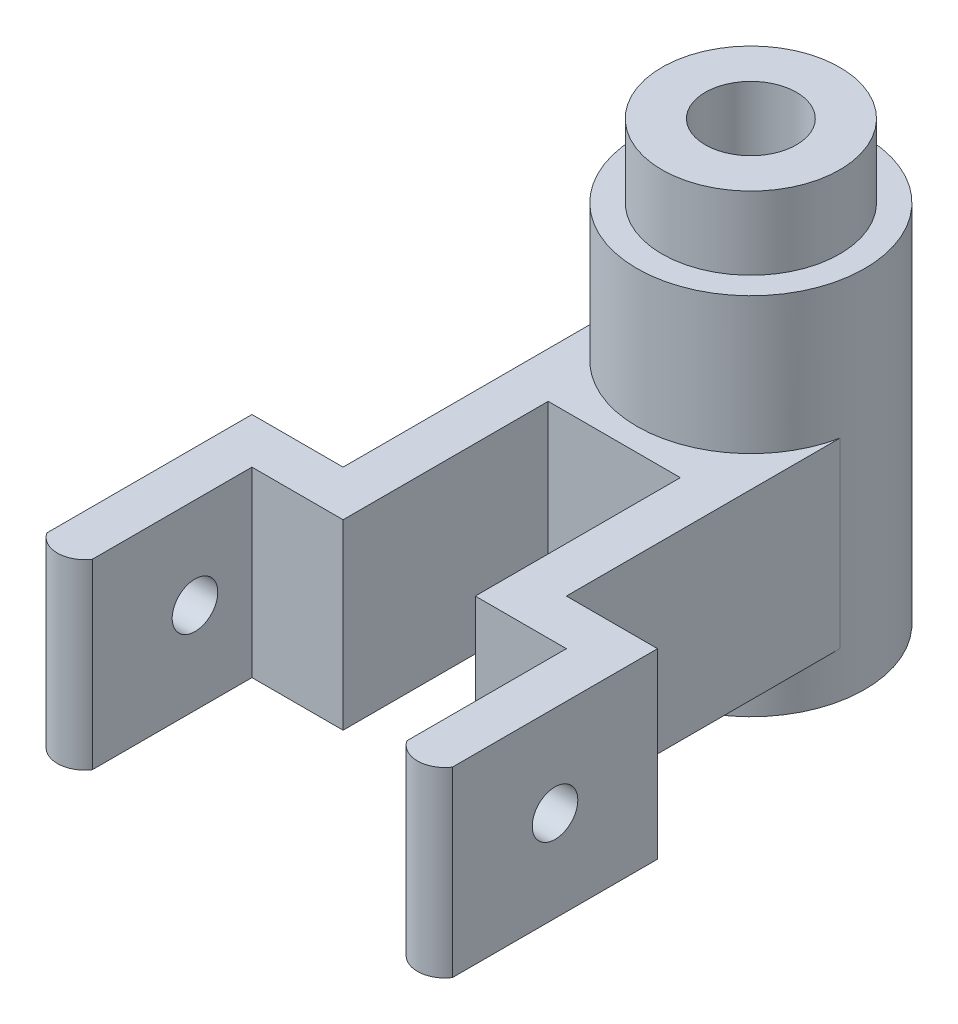
ISO-10303-21;
HEADER;
FILE_DESCRIPTION(('STEP AP214'),'2;1');
FILE_NAME('part.step','',(''),(''),'','','');
FILE_SCHEMA(('AUTOMOTIVE_DESIGN { 1 0 10303 214 1 1 1 1 }'));
ENDSEC;
DATA;
#1=APPLICATION_CONTEXT('core data for automotive mechanical design processes');
#2=APPLICATION_PROTOCOL_DEFINITION('international standard','automotive_design',2000,#1);
#3=PRODUCT_CONTEXT('',#1,'mechanical');
#4=PRODUCT('Part','Part','',(#3));
#5=PRODUCT_RELATED_PRODUCT_CATEGORY('part','',(#4));
#6=PRODUCT_DEFINITION_FORMATION('','',#4);
#7=PRODUCT_DEFINITION_CONTEXT('part definition',#1,'design');
#8=PRODUCT_DEFINITION('design','',#6,#7);
#9=PRODUCT_DEFINITION_SHAPE('','',#8);
#10=(LENGTH_UNIT() NAMED_UNIT(*) SI_UNIT(.MILLI.,.METRE.));
#11=(NAMED_UNIT(*) PLANE_ANGLE_UNIT() SI_UNIT($,.RADIAN.));
#12=(NAMED_UNIT(*) SI_UNIT($,.STERADIAN.) SOLID_ANGLE_UNIT());
#13=UNCERTAINTY_MEASURE_WITH_UNIT(LENGTH_MEASURE(1.E-05),#10,'distance_accuracy_value','');
#14=(GEOMETRIC_REPRESENTATION_CONTEXT(3) GLOBAL_UNCERTAINTY_ASSIGNED_CONTEXT((#13)) GLOBAL_UNIT_ASSIGNED_CONTEXT((#10,
#11,#12)) REPRESENTATION_CONTEXT('',''));
#15=CARTESIAN_POINT('',(0.,0.,0.));
#16=DIRECTION('',(0.,0.,1.));
#17=DIRECTION('',(1.,0.,0.));
#18=AXIS2_PLACEMENT_3D('',#15,#16,#17);
#19=CARTESIAN_POINT('',(0.,80.,0.));
#20=DIRECTION('',(0.,-1.,0.));
#21=DIRECTION('',(0.,0.,-1.));
#22=AXIS2_PLACEMENT_3D('',#19,#20,#21);
#23=CYLINDRICAL_SURFACE('',#22,25.);
#24=DIRECTION('',(0.,-1.,0.));
#25=VECTOR('',#24,1.);
#26=CARTESIAN_POINT('',(-24.5,50.,4.97493718553311));
#27=LINE('',#26,#25);
#28=CARTESIAN_POINT('',(-24.5,50.,4.97493718553311));
#29=VERTEX_POINT('',#28);
#30=CARTESIAN_POINT('',(-24.5,9.99999999999999,4.97493718553311));
#31=VERTEX_POINT('',#30);
#32=EDGE_CURVE('E60',#29,#31,#27,.T.);
#33=ORIENTED_EDGE('',*,*,#32,.F.);
#34=CARTESIAN_POINT('',(0.,50.,0.));
#35=DIRECTION('',(0.,1.,0.));
#36=DIRECTION('',(0.,0.,1.));
#37=AXIS2_PLACEMENT_3D('',#34,#35,#36);
#38=CIRCLE('',#37,25.);
#39=CARTESIAN_POINT('',(24.5,50.,4.97493718553311));
#40=VERTEX_POINT('',#39);
#41=EDGE_CURVE('E63',#29,#40,#38,.T.);
#42=ORIENTED_EDGE('',*,*,#41,.T.);
#43=DIRECTION('',(0.,-1.,0.));
#44=VECTOR('',#43,1.);
#45=CARTESIAN_POINT('',(24.5,50.,4.97493718553311));
#46=LINE('',#45,#44);
#47=CARTESIAN_POINT('',(24.5,10.,4.97493718553311));
#48=VERTEX_POINT('',#47);
#49=EDGE_CURVE('E300',#40,#48,#46,.T.);
#50=ORIENTED_EDGE('',*,*,#49,.T.);
#51=CARTESIAN_POINT('',(0.,9.99999999999999,0.));
#52=DIRECTION('',(0.,1.,0.));
#53=DIRECTION('',(0.,0.,1.));
#54=AXIS2_PLACEMENT_3D('',#51,#52,#53);
#55=CIRCLE('',#54,25.);
#56=EDGE_CURVE('E303',#31,#48,#55,.T.);
#57=ORIENTED_EDGE('',*,*,#56,.F.);
#58=EDGE_LOOP('',(#33,#42,#50,#57));
#59=FACE_BOUND('',#58,.T.);
#60=CARTESIAN_POINT('',(0.,80.,0.));
#61=DIRECTION('',(0.,1.,0.));
#62=DIRECTION('',(0.,0.,1.));
#63=AXIS2_PLACEMENT_3D('',#60,#61,#62);
#64=CIRCLE('',#63,25.);
#65=CARTESIAN_POINT('',(0.,80.,25.));
#66=VERTEX_POINT('',#65);
#67=EDGE_CURVE('E321',#66,#66,#64,.T.);
#68=ORIENTED_EDGE('',*,*,#67,.F.);
#69=EDGE_LOOP('',(#68));
#70=FACE_BOUND('',#69,.T.);
#71=CARTESIAN_POINT('',(0.,0.,0.));
#72=DIRECTION('',(0.,1.,0.));
#73=DIRECTION('',(0.,0.,1.));
#74=AXIS2_PLACEMENT_3D('',#71,#72,#73);
#75=CIRCLE('',#74,25.);
#76=CARTESIAN_POINT('',(0.,0.,25.));
#77=VERTEX_POINT('',#76);
#78=EDGE_CURVE('E316',#77,#77,#75,.T.);
#79=ORIENTED_EDGE('',*,*,#78,.T.);
#80=EDGE_LOOP('',(#79));
#81=FACE_BOUND('',#80,.T.);
#82=ADVANCED_FACE('F43',(#59,#70,#81),#23,.T.);
#83=CARTESIAN_POINT('',(0.,80.,0.));
#84=DIRECTION('',(0.,1.,0.));
#85=DIRECTION('',(0.,0.,1.));
#86=AXIS2_PLACEMENT_3D('',#83,#84,#85);
#87=PLANE('',#86);
#88=CARTESIAN_POINT('',(0.,80.,0.));
#89=DIRECTION('',(0.,1.,0.));
#90=DIRECTION('',(0.,0.,1.));
#91=AXIS2_PLACEMENT_3D('',#88,#89,#90);
#92=CIRCLE('',#91,19.5);
#93=CARTESIAN_POINT('',(0.,80.,19.5));
#94=VERTEX_POINT('',#93);
#95=EDGE_CURVE('E320',#94,#94,#92,.T.);
#96=ORIENTED_EDGE('',*,*,#95,.F.);
#97=EDGE_LOOP('',(#96));
#98=FACE_BOUND('',#97,.T.);
#99=ORIENTED_EDGE('',*,*,#67,.T.);
#100=EDGE_LOOP('',(#99));
#101=FACE_BOUND('',#100,.T.);
#102=ADVANCED_FACE('F356',(#98,#101),#87,.T.);
#103=CARTESIAN_POINT('',(0.,0.,0.));
#104=DIRECTION('',(0.,1.,0.));
#105=DIRECTION('',(0.,0.,1.));
#106=AXIS2_PLACEMENT_3D('',#103,#104,#105);
#107=PLANE('',#106);
#108=CARTESIAN_POINT('',(0.,0.,0.));
#109=DIRECTION('',(0.,1.,0.));
#110=DIRECTION('',(0.,0.,1.));
#111=AXIS2_PLACEMENT_3D('',#108,#109,#110);
#112=CIRCLE('',#111,10.);
#113=CARTESIAN_POINT('',(0.,0.,10.));
#114=VERTEX_POINT('',#113);
#115=EDGE_CURVE('E306',#114,#114,#112,.T.);
#116=ORIENTED_EDGE('',*,*,#115,.T.);
#117=EDGE_LOOP('',(#116));
#118=FACE_BOUND('',#117,.T.);
#119=ORIENTED_EDGE('',*,*,#78,.F.);
#120=EDGE_LOOP('',(#119));
#121=FACE_BOUND('',#120,.T.);
#122=ADVANCED_FACE('F362',(#118,#121),#107,.F.);
#123=CARTESIAN_POINT('',(0.,96.,0.));
#124=DIRECTION('',(0.,-1.,0.));
#125=DIRECTION('',(0.,0.,-1.));
#126=AXIS2_PLACEMENT_3D('',#123,#124,#125);
#127=CYLINDRICAL_SURFACE('',#126,19.5);
#128=CARTESIAN_POINT('',(0.,96.,0.));
#129=DIRECTION('',(0.,1.,0.));
#130=DIRECTION('',(0.,0.,1.));
#131=AXIS2_PLACEMENT_3D('',#128,#129,#130);
#132=CIRCLE('',#131,19.5);
#133=CARTESIAN_POINT('',(0.,96.,19.5));
#134=VERTEX_POINT('',#133);
#135=EDGE_CURVE('E313',#134,#134,#132,.T.);
#136=ORIENTED_EDGE('',*,*,#135,.F.);
#137=EDGE_LOOP('',(#136));
#138=FACE_BOUND('',#137,.T.);
#139=ORIENTED_EDGE('',*,*,#95,.T.);
#140=EDGE_LOOP('',(#139));
#141=FACE_BOUND('',#140,.T.);
#142=ADVANCED_FACE('F371',(#138,#141),#127,.T.);
#143=CARTESIAN_POINT('',(0.,96.,0.));
#144=DIRECTION('',(0.,1.,0.));
#145=DIRECTION('',(0.,0.,1.));
#146=AXIS2_PLACEMENT_3D('',#143,#144,#145);
#147=PLANE('',#146);
#148=CARTESIAN_POINT('',(0.,96.,0.));
#149=DIRECTION('',(0.,1.,0.));
#150=DIRECTION('',(0.,0.,1.));
#151=AXIS2_PLACEMENT_3D('',#148,#149,#150);
#152=CIRCLE('',#151,10.);
#153=CARTESIAN_POINT('',(0.,96.,10.));
#154=VERTEX_POINT('',#153);
#155=EDGE_CURVE('E307',#154,#154,#152,.T.);
#156=ORIENTED_EDGE('',*,*,#155,.F.);
#157=EDGE_LOOP('',(#156));
#158=FACE_BOUND('',#157,.T.);
#159=ORIENTED_EDGE('',*,*,#135,.T.);
#160=EDGE_LOOP('',(#159));
#161=FACE_BOUND('',#160,.T.);
#162=ADVANCED_FACE('F376',(#158,#161),#147,.T.);
#163=CARTESIAN_POINT('',(0.,0.,0.));
#164=DIRECTION('',(0.,1.,0.));
#165=DIRECTION('',(0.,0.,1.));
#166=AXIS2_PLACEMENT_3D('',#163,#164,#165);
#167=CYLINDRICAL_SURFACE('',#166,10.);
#168=DIRECTION('',(0.,1.,0.));
#169=VECTOR('',#168,1.);
#170=CARTESIAN_POINT('',(8.67467578644873,0.,4.97493718553311));
#171=LINE('',#170,#169);
#172=CARTESIAN_POINT('',(8.67467578644873,50.,4.97493718553311));
#173=VERTEX_POINT('',#172);
#174=CARTESIAN_POINT('',(8.67467578644873,10.,4.97493718553311));
#175=VERTEX_POINT('',#174);
#176=EDGE_CURVE('E49',#173,#175,#171,.F.);
#177=ORIENTED_EDGE('',*,*,#176,.F.);
#178=CARTESIAN_POINT('',(0.,50.,0.));
#179=DIRECTION('',(0.,1.,0.));
#180=DIRECTION('',(0.,0.,1.));
#181=AXIS2_PLACEMENT_3D('',#178,#179,#180);
#182=CIRCLE('',#181,10.);
#183=CARTESIAN_POINT('',(-8.67467578644873,50.,4.97493718553311));
#184=VERTEX_POINT('',#183);
#185=EDGE_CURVE('E11',#173,#184,#182,.F.);
#186=ORIENTED_EDGE('',*,*,#185,.T.);
#187=DIRECTION('',(0.,1.,0.));
#188=VECTOR('',#187,1.);
#189=CARTESIAN_POINT('',(-8.67467578644873,0.,4.97493718553311));
#190=LINE('',#189,#188);
#191=CARTESIAN_POINT('',(-8.67467578644873,10.,4.97493718553311));
#192=VERTEX_POINT('',#191);
#193=EDGE_CURVE('E327',#192,#184,#190,.T.);
#194=ORIENTED_EDGE('',*,*,#193,.F.);
#195=CARTESIAN_POINT('',(0.,10.,0.));
#196=DIRECTION('',(0.,1.,0.));
#197=DIRECTION('',(0.,0.,1.));
#198=AXIS2_PLACEMENT_3D('',#195,#196,#197);
#199=CIRCLE('',#198,10.);
#200=EDGE_CURVE('E319',#175,#192,#199,.F.);
#201=ORIENTED_EDGE('',*,*,#200,.F.);
#202=EDGE_LOOP('',(#177,#186,#194,#201));
#203=FACE_BOUND('',#202,.T.);
#204=ORIENTED_EDGE('',*,*,#115,.F.);
#205=EDGE_LOOP('',(#204));
#206=FACE_BOUND('',#205,.T.);
#207=ORIENTED_EDGE('',*,*,#155,.T.);
#208=EDGE_LOOP('',(#207));
#209=FACE_BOUND('',#208,.T.);
#210=ADVANCED_FACE('F337',(#203,#206,#209),#167,.F.);
#211=CARTESIAN_POINT('',(0.,10.,0.));
#212=DIRECTION('',(0.,1.,0.));
#213=DIRECTION('',(0.,0.,1.));
#214=AXIS2_PLACEMENT_3D('',#211,#212,#213);
#215=PLANE('',#214);
#216=DIRECTION('',(-1.,0.,0.));
#217=VECTOR('',#216,1.);
#218=CARTESIAN_POINT('',(-24.5,10.,4.97493718553311));
#219=LINE('',#218,#217);
#220=EDGE_CURVE('E284',#175,#192,#219,.T.);
#221=ORIENTED_EDGE('',*,*,#220,.F.);
#222=ORIENTED_EDGE('',*,*,#200,.T.);
#223=EDGE_LOOP('',(#221,#222));
#224=FACE_BOUND('',#223,.T.);
#225=ADVANCED_FACE('F336',(#224),#215,.F.);
#226=CARTESIAN_POINT('',(0.,50.,0.));
#227=DIRECTION('',(0.,1.,0.));
#228=DIRECTION('',(0.,0.,1.));
#229=AXIS2_PLACEMENT_3D('',#226,#227,#228);
#230=PLANE('',#229);
#231=ORIENTED_EDGE('',*,*,#185,.F.);
#232=DIRECTION('',(-1.,0.,0.));
#233=VECTOR('',#232,1.);
#234=CARTESIAN_POINT('',(-24.5,50.,4.97493718553311));
#235=LINE('',#234,#233);
#236=EDGE_CURVE('E290',#173,#184,#235,.T.);
#237=ORIENTED_EDGE('',*,*,#236,.T.);
#238=EDGE_LOOP('',(#231,#237));
#239=FACE_BOUND('',#238,.T.);
#240=ADVANCED_FACE('F345',(#239),#230,.T.);
#241=CARTESIAN_POINT('',(-24.5,50.,4.97493718553311));
#242=DIRECTION('',(0.,0.,1.));
#243=DIRECTION('',(1.,0.,0.));
#244=AXIS2_PLACEMENT_3D('',#241,#242,#243);
#245=PLANE('',#244);
#246=ORIENTED_EDGE('',*,*,#236,.F.);
#247=ORIENTED_EDGE('',*,*,#176,.T.);
#248=ORIENTED_EDGE('',*,*,#220,.T.);
#249=ORIENTED_EDGE('',*,*,#193,.T.);
#250=EDGE_LOOP('',(#246,#247,#248,#249));
#251=FACE_BOUND('',#250,.T.);
#252=ADVANCED_FACE('F331',(#251),#245,.F.);
#253=DIRECTION('',(0.,0.,1.));
#254=VECTOR('',#253,1.);
#255=CARTESIAN_POINT('',(-14.5,50.,64.9749371855331));
#256=LINE('',#255,#254);
#257=CARTESIAN_POINT('',(-14.5,50.,29.9749371855331));
#258=VERTEX_POINT('',#257);
#259=CARTESIAN_POINT('',(-14.5,50.,74.9749371855331));
#260=VERTEX_POINT('',#259);
#261=EDGE_CURVE('E251',#258,#260,#256,.T.);
#262=ORIENTED_EDGE('',*,*,#261,.F.);
#263=DIRECTION('',(-1.,0.,0.));
#264=VECTOR('',#263,1.);
#265=CARTESIAN_POINT('',(-14.5,50.,29.9749371855331));
#266=LINE('',#265,#264);
#267=CARTESIAN_POINT('',(14.5,50.,29.9749371855331));
#268=VERTEX_POINT('',#267);
#269=EDGE_CURVE('E266',#268,#258,#266,.T.);
#270=ORIENTED_EDGE('',*,*,#269,.F.);
#271=DIRECTION('',(0.,0.,-1.));
#272=VECTOR('',#271,1.);
#273=CARTESIAN_POINT('',(14.5,50.,64.9749371855331));
#274=LINE('',#273,#272);
#275=CARTESIAN_POINT('',(14.5,50.,74.9749371855331));
#276=VERTEX_POINT('',#275);
#277=EDGE_CURVE('E272',#276,#268,#274,.T.);
#278=ORIENTED_EDGE('',*,*,#277,.F.);
#279=DIRECTION('',(1.,0.,0.));
#280=VECTOR('',#279,1.);
#281=CARTESIAN_POINT('',(14.5,50.,74.9749371855331));
#282=LINE('',#281,#280);
#283=CARTESIAN_POINT('',(34.5,50.,74.9749371855331));
#284=VERTEX_POINT('',#283);
#285=EDGE_CURVE('E220',#276,#284,#282,.T.);
#286=ORIENTED_EDGE('',*,*,#285,.T.);
#287=DIRECTION('',(0.,0.,1.));
#288=VECTOR('',#287,1.);
#289=CARTESIAN_POINT('',(34.5,50.,74.9749371855331));
#290=LINE('',#289,#288);
#291=CARTESIAN_POINT('',(34.5,50.,109.974937185533));
#292=VERTEX_POINT('',#291);
#293=EDGE_CURVE('E238',#284,#292,#290,.T.);
#294=ORIENTED_EDGE('',*,*,#293,.T.);
#295=CARTESIAN_POINT('',(39.5,50.,106.658312395178));
#296=DIRECTION('',(0.,1.,0.));
#297=DIRECTION('',(0.,0.,1.));
#298=AXIS2_PLACEMENT_3D('',#295,#296,#297);
#299=CIRCLE('',#298,5.99999999999999);
#300=CARTESIAN_POINT('',(44.5,50.,109.974937185533));
#301=VERTEX_POINT('',#300);
#302=EDGE_CURVE('E241',#292,#301,#299,.T.);
#303=ORIENTED_EDGE('',*,*,#302,.T.);
#304=DIRECTION('',(0.,0.,-1.));
#305=VECTOR('',#304,1.);
#306=CARTESIAN_POINT('',(44.5,50.,64.9749371855331));
#307=LINE('',#306,#305);
#308=CARTESIAN_POINT('',(44.5,50.,64.9749371855331));
#309=VERTEX_POINT('',#308);
#310=EDGE_CURVE('E246',#301,#309,#307,.T.);
#311=ORIENTED_EDGE('',*,*,#310,.T.);
#312=DIRECTION('',(-1.,0.,0.));
#313=VECTOR('',#312,1.);
#314=CARTESIAN_POINT('',(14.5,50.,64.9749371855331));
#315=LINE('',#314,#313);
#316=CARTESIAN_POINT('',(24.5,50.,64.9749371855331));
#317=VERTEX_POINT('',#316);
#318=EDGE_CURVE('E230',#309,#317,#315,.T.);
#319=ORIENTED_EDGE('',*,*,#318,.T.);
#320=DIRECTION('',(0.,0.,-1.));
#321=VECTOR('',#320,1.);
#322=CARTESIAN_POINT('',(24.5,50.,4.97493718553311));
#323=LINE('',#322,#321);
#324=EDGE_CURVE('E282',#317,#40,#323,.T.);
#325=ORIENTED_EDGE('',*,*,#324,.T.);
#326=ORIENTED_EDGE('',*,*,#41,.F.);
#327=DIRECTION('',(0.,0.,1.));
#328=VECTOR('',#327,1.);
#329=CARTESIAN_POINT('',(-24.5,50.,4.97493718553311));
#330=LINE('',#329,#328);
#331=CARTESIAN_POINT('',(-24.5,50.,64.9749371855331));
#332=VERTEX_POINT('',#331);
#333=EDGE_CURVE('E285',#29,#332,#330,.T.);
#334=ORIENTED_EDGE('',*,*,#333,.T.);
#335=DIRECTION('',(-1.,0.,0.));
#336=VECTOR('',#335,1.);
#337=CARTESIAN_POINT('',(-14.5,50.,64.9749371855331));
#338=LINE('',#337,#336);
#339=CARTESIAN_POINT('',(-44.5,50.,64.9749371855331));
#340=VERTEX_POINT('',#339);
#341=EDGE_CURVE('E205',#332,#340,#338,.T.);
#342=ORIENTED_EDGE('',*,*,#341,.T.);
#343=DIRECTION('',(0.,0.,1.));
#344=VECTOR('',#343,1.);
#345=CARTESIAN_POINT('',(-44.5,50.,74.9749371855331));
#346=LINE('',#345,#344);
#347=CARTESIAN_POINT('',(-44.5,50.,109.974937185533));
#348=VERTEX_POINT('',#347);
#349=EDGE_CURVE('E181',#340,#348,#346,.T.);
#350=ORIENTED_EDGE('',*,*,#349,.T.);
#351=CARTESIAN_POINT('',(-39.5,50.,106.658312395178));
#352=DIRECTION('',(0.,1.,0.));
#353=DIRECTION('',(0.,0.,1.));
#354=AXIS2_PLACEMENT_3D('',#351,#352,#353);
#355=CIRCLE('',#354,6.);
#356=CARTESIAN_POINT('',(-34.5,50.,109.974937185533));
#357=VERTEX_POINT('',#356);
#358=EDGE_CURVE('E206',#348,#357,#355,.T.);
#359=ORIENTED_EDGE('',*,*,#358,.T.);
#360=DIRECTION('',(0.,0.,-1.));
#361=VECTOR('',#360,1.);
#362=CARTESIAN_POINT('',(-34.5,50.,74.9749371855331));
#363=LINE('',#362,#361);
#364=CARTESIAN_POINT('',(-34.5,50.,74.9749371855331));
#365=VERTEX_POINT('',#364);
#366=EDGE_CURVE('E207',#357,#365,#363,.T.);
#367=ORIENTED_EDGE('',*,*,#366,.T.);
#368=DIRECTION('',(1.,0.,0.));
#369=VECTOR('',#368,1.);
#370=CARTESIAN_POINT('',(-14.5,50.,74.9749371855331));
#371=LINE('',#370,#369);
#372=EDGE_CURVE('E176',#365,#260,#371,.T.);
#373=ORIENTED_EDGE('',*,*,#372,.T.);
#374=EDGE_LOOP('',(#262,#270,#278,#286,#294,#303,#311,#319,#325,#326,#334,#342,#350,#359,#367,#373));
#375=FACE_BOUND('',#374,.T.);
#376=ADVANCED_FACE('F344',(#375),#230,.T.);
#377=DIRECTION('',(-1.,0.,0.));
#378=VECTOR('',#377,1.);
#379=CARTESIAN_POINT('',(-14.5,10.,29.9749371855331));
#380=LINE('',#379,#378);
#381=CARTESIAN_POINT('',(14.5,10.,29.9749371855331));
#382=VERTEX_POINT('',#381);
#383=CARTESIAN_POINT('',(-14.5,10.,29.9749371855331));
#384=VERTEX_POINT('',#383);
#385=EDGE_CURVE('E267',#382,#384,#380,.T.);
#386=ORIENTED_EDGE('',*,*,#385,.T.);
#387=DIRECTION('',(0.,0.,1.));
#388=VECTOR('',#387,1.);
#389=CARTESIAN_POINT('',(-14.5,10.,64.9749371855331));
#390=LINE('',#389,#388);
#391=CARTESIAN_POINT('',(-14.5,10.,74.9749371855331));
#392=VERTEX_POINT('',#391);
#393=EDGE_CURVE('E263',#384,#392,#390,.T.);
#394=ORIENTED_EDGE('',*,*,#393,.T.);
#395=DIRECTION('',(1.,0.,0.));
#396=VECTOR('',#395,1.);
#397=CARTESIAN_POINT('',(-14.5,10.,74.9749371855331));
#398=LINE('',#397,#396);
#399=CARTESIAN_POINT('',(-34.5,10.,74.9749371855331));
#400=VERTEX_POINT('',#399);
#401=EDGE_CURVE('E183',#400,#392,#398,.T.);
#402=ORIENTED_EDGE('',*,*,#401,.F.);
#403=DIRECTION('',(0.,0.,-1.));
#404=VECTOR('',#403,1.);
#405=CARTESIAN_POINT('',(-34.5,10.,74.9749371855331));
#406=LINE('',#405,#404);
#407=CARTESIAN_POINT('',(-34.5,10.,109.974937185533));
#408=VERTEX_POINT('',#407);
#409=EDGE_CURVE('E192',#408,#400,#406,.T.);
#410=ORIENTED_EDGE('',*,*,#409,.F.);
#411=CARTESIAN_POINT('',(-39.5,10.,106.658312395178));
#412=DIRECTION('',(0.,1.,0.));
#413=DIRECTION('',(0.,0.,1.));
#414=AXIS2_PLACEMENT_3D('',#411,#412,#413);
#415=CIRCLE('',#414,6.);
#416=CARTESIAN_POINT('',(-44.5,10.,109.974937185533));
#417=VERTEX_POINT('',#416);
#418=EDGE_CURVE('E195',#417,#408,#415,.T.);
#419=ORIENTED_EDGE('',*,*,#418,.F.);
#420=DIRECTION('',(0.,0.,1.));
#421=VECTOR('',#420,1.);
#422=CARTESIAN_POINT('',(-44.5,10.,64.9749371855331));
#423=LINE('',#422,#421);
#424=CARTESIAN_POINT('',(-44.5,10.,64.9749371855331));
#425=VERTEX_POINT('',#424);
#426=EDGE_CURVE('E174',#425,#417,#423,.T.);
#427=ORIENTED_EDGE('',*,*,#426,.F.);
#428=DIRECTION('',(-1.,0.,0.));
#429=VECTOR('',#428,1.);
#430=CARTESIAN_POINT('',(-14.5,10.,64.9749371855331));
#431=LINE('',#430,#429);
#432=CARTESIAN_POINT('',(-24.5,10.,64.9749371855331));
#433=VERTEX_POINT('',#432);
#434=EDGE_CURVE('E164',#433,#425,#431,.T.);
#435=ORIENTED_EDGE('',*,*,#434,.F.);
#436=DIRECTION('',(0.,0.,1.));
#437=VECTOR('',#436,1.);
#438=CARTESIAN_POINT('',(-24.5,10.,4.97493718553311));
#439=LINE('',#438,#437);
#440=EDGE_CURVE('E278',#31,#433,#439,.T.);
#441=ORIENTED_EDGE('',*,*,#440,.F.);
#442=ORIENTED_EDGE('',*,*,#56,.T.);
#443=DIRECTION('',(0.,0.,-1.));
#444=VECTOR('',#443,1.);
#445=CARTESIAN_POINT('',(24.5,10.,4.97493718553311));
#446=LINE('',#445,#444);
#447=CARTESIAN_POINT('',(24.5,10.,64.9749371855331));
#448=VERTEX_POINT('',#447);
#449=EDGE_CURVE('E292',#448,#48,#446,.T.);
#450=ORIENTED_EDGE('',*,*,#449,.F.);
#451=DIRECTION('',(-1.,0.,0.));
#452=VECTOR('',#451,1.);
#453=CARTESIAN_POINT('',(14.5,10.,64.9749371855331));
#454=LINE('',#453,#452);
#455=CARTESIAN_POINT('',(44.5,10.,64.9749371855331));
#456=VERTEX_POINT('',#455);
#457=EDGE_CURVE('E234',#456,#448,#454,.T.);
#458=ORIENTED_EDGE('',*,*,#457,.F.);
#459=DIRECTION('',(0.,0.,-1.));
#460=VECTOR('',#459,1.);
#461=CARTESIAN_POINT('',(44.5,10.,74.9749371855331));
#462=LINE('',#461,#460);
#463=CARTESIAN_POINT('',(44.5,10.,109.974937185533));
#464=VERTEX_POINT('',#463);
#465=EDGE_CURVE('E233',#464,#456,#462,.T.);
#466=ORIENTED_EDGE('',*,*,#465,.F.);
#467=CARTESIAN_POINT('',(39.5,10.,106.658312395178));
#468=DIRECTION('',(0.,1.,0.));
#469=DIRECTION('',(0.,0.,1.));
#470=AXIS2_PLACEMENT_3D('',#467,#468,#469);
#471=CIRCLE('',#470,5.99999999999999);
#472=CARTESIAN_POINT('',(34.5,10.,109.974937185533));
#473=VERTEX_POINT('',#472);
#474=EDGE_CURVE('E229',#473,#464,#471,.T.);
#475=ORIENTED_EDGE('',*,*,#474,.F.);
#476=DIRECTION('',(0.,0.,1.));
#477=VECTOR('',#476,1.);
#478=CARTESIAN_POINT('',(34.5,10.,74.9749371855331));
#479=LINE('',#478,#477);
#480=CARTESIAN_POINT('',(34.5,10.,74.9749371855331));
#481=VERTEX_POINT('',#480);
#482=EDGE_CURVE('E228',#481,#473,#479,.T.);
#483=ORIENTED_EDGE('',*,*,#482,.F.);
#484=DIRECTION('',(1.,0.,0.));
#485=VECTOR('',#484,1.);
#486=CARTESIAN_POINT('',(14.5,10.,74.9749371855331));
#487=LINE('',#486,#485);
#488=CARTESIAN_POINT('',(14.5,10.,74.9749371855331));
#489=VERTEX_POINT('',#488);
#490=EDGE_CURVE('E224',#489,#481,#487,.T.);
#491=ORIENTED_EDGE('',*,*,#490,.F.);
#492=DIRECTION('',(0.,0.,-1.));
#493=VECTOR('',#492,1.);
#494=CARTESIAN_POINT('',(14.5,10.,64.9749371855331));
#495=LINE('',#494,#493);
#496=EDGE_CURVE('E264',#489,#382,#495,.T.);
#497=ORIENTED_EDGE('',*,*,#496,.T.);
#498=EDGE_LOOP('',(#386,#394,#402,#410,#419,#427,#435,#441,#442,#450,#458,#466,#475,#483,#491,#497));
#499=FACE_BOUND('',#498,.T.);
#500=ADVANCED_FACE('F187',(#499),#215,.F.);
#501=CARTESIAN_POINT('',(-24.5,50.,4.97493718553311));
#502=DIRECTION('',(1.,0.,0.));
#503=DIRECTION('',(0.,0.,-1.));
#504=AXIS2_PLACEMENT_3D('',#501,#502,#503);
#505=PLANE('',#504);
#506=ORIENTED_EDGE('',*,*,#440,.T.);
#507=DIRECTION('',(0.,-1.,0.));
#508=VECTOR('',#507,1.);
#509=CARTESIAN_POINT('',(-24.5,50.,64.9749371855331));
#510=LINE('',#509,#508);
#511=EDGE_CURVE('E173',#332,#433,#510,.T.);
#512=ORIENTED_EDGE('',*,*,#511,.F.);
#513=ORIENTED_EDGE('',*,*,#333,.F.);
#514=ORIENTED_EDGE('',*,*,#32,.T.);
#515=EDGE_LOOP('',(#506,#512,#513,#514));
#516=FACE_BOUND('',#515,.T.);
#517=ADVANCED_FACE('F383',(#516),#505,.F.);
#518=CARTESIAN_POINT('',(24.5,50.,4.97493718553311));
#519=DIRECTION('',(-1.,0.,0.));
#520=DIRECTION('',(0.,0.,1.));
#521=AXIS2_PLACEMENT_3D('',#518,#519,#520);
#522=PLANE('',#521);
#523=ORIENTED_EDGE('',*,*,#449,.T.);
#524=ORIENTED_EDGE('',*,*,#49,.F.);
#525=ORIENTED_EDGE('',*,*,#324,.F.);
#526=DIRECTION('',(0.,-1.,0.));
#527=VECTOR('',#526,1.);
#528=CARTESIAN_POINT('',(24.5,50.,64.9749371855331));
#529=LINE('',#528,#527);
#530=EDGE_CURVE('E297',#317,#448,#529,.T.);
#531=ORIENTED_EDGE('',*,*,#530,.T.);
#532=EDGE_LOOP('',(#523,#524,#525,#531));
#533=FACE_BOUND('',#532,.T.);
#534=ADVANCED_FACE('F390',(#533),#522,.F.);
#535=CARTESIAN_POINT('',(-14.5,10.,64.9749371855331));
#536=DIRECTION('',(-1.,0.,0.));
#537=DIRECTION('',(0.,0.,1.));
#538=AXIS2_PLACEMENT_3D('',#535,#536,#537);
#539=PLANE('',#538);
#540=ORIENTED_EDGE('',*,*,#261,.T.);
#541=DIRECTION('',(0.,1.,0.));
#542=VECTOR('',#541,1.);
#543=CARTESIAN_POINT('',(-14.5,10.,74.9749371855331));
#544=LINE('',#543,#542);
#545=EDGE_CURVE('E212',#392,#260,#544,.T.);
#546=ORIENTED_EDGE('',*,*,#545,.F.);
#547=ORIENTED_EDGE('',*,*,#393,.F.);
#548=DIRECTION('',(0.,1.,0.));
#549=VECTOR('',#548,1.);
#550=CARTESIAN_POINT('',(-14.5,10.,29.9749371855331));
#551=LINE('',#550,#549);
#552=EDGE_CURVE('E279',#384,#258,#551,.T.);
#553=ORIENTED_EDGE('',*,*,#552,.T.);
#554=EDGE_LOOP('',(#540,#546,#547,#553));
#555=FACE_BOUND('',#554,.T.);
#556=ADVANCED_FACE('F388',(#555),#539,.F.);
#557=CARTESIAN_POINT('',(-14.5,10.,29.9749371855331));
#558=DIRECTION('',(0.,0.,-1.));
#559=DIRECTION('',(-1.,0.,0.));
#560=AXIS2_PLACEMENT_3D('',#557,#558,#559);
#561=PLANE('',#560);
#562=ORIENTED_EDGE('',*,*,#269,.T.);
#563=ORIENTED_EDGE('',*,*,#552,.F.);
#564=ORIENTED_EDGE('',*,*,#385,.F.);
#565=DIRECTION('',(0.,1.,0.));
#566=VECTOR('',#565,1.);
#567=CARTESIAN_POINT('',(14.5,10.,29.9749371855331));
#568=LINE('',#567,#566);
#569=EDGE_CURVE('E271',#382,#268,#568,.T.);
#570=ORIENTED_EDGE('',*,*,#569,.T.);
#571=EDGE_LOOP('',(#562,#563,#564,#570));
#572=FACE_BOUND('',#571,.T.);
#573=ADVANCED_FACE('F417',(#572),#561,.F.);
#574=CARTESIAN_POINT('',(14.5,10.,64.9749371855331));
#575=DIRECTION('',(1.,0.,0.));
#576=DIRECTION('',(0.,0.,-1.));
#577=AXIS2_PLACEMENT_3D('',#574,#575,#576);
#578=PLANE('',#577);
#579=ORIENTED_EDGE('',*,*,#277,.T.);
#580=ORIENTED_EDGE('',*,*,#569,.F.);
#581=ORIENTED_EDGE('',*,*,#496,.F.);
#582=DIRECTION('',(0.,1.,0.));
#583=VECTOR('',#582,1.);
#584=CARTESIAN_POINT('',(14.5,10.,74.9749371855331));
#585=LINE('',#584,#583);
#586=EDGE_CURVE('E240',#489,#276,#585,.T.);
#587=ORIENTED_EDGE('',*,*,#586,.T.);
#588=EDGE_LOOP('',(#579,#580,#581,#587));
#589=FACE_BOUND('',#588,.T.);
#590=ADVANCED_FACE('F425',(#589),#578,.F.);
#591=CARTESIAN_POINT('',(14.5,10.,64.9749371855331));
#592=DIRECTION('',(0.,0.,-1.));
#593=DIRECTION('',(-1.,0.,0.));
#594=AXIS2_PLACEMENT_3D('',#591,#592,#593);
#595=PLANE('',#594);
#596=ORIENTED_EDGE('',*,*,#530,.F.);
#597=ORIENTED_EDGE('',*,*,#318,.F.);
#598=DIRECTION('',(0.,1.,0.));
#599=VECTOR('',#598,1.);
#600=CARTESIAN_POINT('',(44.5,10.,64.9749371855331));
#601=LINE('',#600,#599);
#602=EDGE_CURVE('E253',#456,#309,#601,.T.);
#603=ORIENTED_EDGE('',*,*,#602,.F.);
#604=ORIENTED_EDGE('',*,*,#457,.T.);
#605=EDGE_LOOP('',(#596,#597,#603,#604));
#606=FACE_BOUND('',#605,.T.);
#607=ADVANCED_FACE('F422',(#606),#595,.T.);
#608=CARTESIAN_POINT('',(44.5,10.,64.9749371855331));
#609=DIRECTION('',(1.,0.,0.));
#610=DIRECTION('',(0.,0.,-1.));
#611=AXIS2_PLACEMENT_3D('',#608,#609,#610);
#612=PLANE('',#611);
#613=CARTESIAN_POINT('',(44.5,30.,87.4749371855331));
#614=DIRECTION('',(1.,0.,0.));
#615=DIRECTION('',(0.,0.,-1.));
#616=AXIS2_PLACEMENT_3D('',#613,#614,#615);
#617=CIRCLE('',#616,5.);
#618=CARTESIAN_POINT('',(44.5,30.,82.4749371855331));
#619=VERTEX_POINT('',#618);
#620=EDGE_CURVE('E677',#619,#619,#617,.T.);
#621=ORIENTED_EDGE('',*,*,#620,.F.);
#622=EDGE_LOOP('',(#621));
#623=FACE_BOUND('',#622,.T.);
#624=ORIENTED_EDGE('',*,*,#310,.F.);
#625=DIRECTION('',(0.,1.,0.));
#626=VECTOR('',#625,1.);
#627=CARTESIAN_POINT('',(44.5,10.,109.974937185533));
#628=LINE('',#627,#626);
#629=EDGE_CURVE('E255',#464,#301,#628,.T.);
#630=ORIENTED_EDGE('',*,*,#629,.F.);
#631=ORIENTED_EDGE('',*,*,#465,.T.);
#632=ORIENTED_EDGE('',*,*,#602,.T.);
#633=EDGE_LOOP('',(#624,#630,#631,#632));
#634=FACE_BOUND('',#633,.T.);
#635=ADVANCED_FACE('F432',(#623,#634),#612,.T.);
#636=CARTESIAN_POINT('',(39.5,10.,106.658312395178));
#637=DIRECTION('',(0.,1.,0.));
#638=DIRECTION('',(0.,0.,1.));
#639=AXIS2_PLACEMENT_3D('',#636,#637,#638);
#640=CYLINDRICAL_SURFACE('',#639,5.99999999999999);
#641=ORIENTED_EDGE('',*,*,#302,.F.);
#642=DIRECTION('',(0.,1.,0.));
#643=VECTOR('',#642,1.);
#644=CARTESIAN_POINT('',(34.5,10.,109.974937185533));
#645=LINE('',#644,#643);
#646=EDGE_CURVE('E260',#473,#292,#645,.T.);
#647=ORIENTED_EDGE('',*,*,#646,.F.);
#648=ORIENTED_EDGE('',*,*,#474,.T.);
#649=ORIENTED_EDGE('',*,*,#629,.T.);
#650=EDGE_LOOP('',(#641,#647,#648,#649));
#651=FACE_BOUND('',#650,.T.);
#652=ADVANCED_FACE('F442',(#651),#640,.T.);
#653=CARTESIAN_POINT('',(34.5,10.,74.9749371855331));
#654=DIRECTION('',(-1.,0.,0.));
#655=DIRECTION('',(0.,0.,1.));
#656=AXIS2_PLACEMENT_3D('',#653,#654,#655);
#657=PLANE('',#656);
#658=CARTESIAN_POINT('',(34.5,30.,87.4749371855331));
#659=DIRECTION('',(-1.,0.,0.));
#660=DIRECTION('',(0.,0.,1.));
#661=AXIS2_PLACEMENT_3D('',#658,#659,#660);
#662=CIRCLE('',#661,5.);
#663=CARTESIAN_POINT('',(34.5,30.,92.4749371855331));
#664=VERTEX_POINT('',#663);
#665=EDGE_CURVE('E204',#664,#664,#662,.T.);
#666=ORIENTED_EDGE('',*,*,#665,.F.);
#667=EDGE_LOOP('',(#666));
#668=FACE_BOUND('',#667,.T.);
#669=ORIENTED_EDGE('',*,*,#293,.F.);
#670=DIRECTION('',(0.,1.,0.));
#671=VECTOR('',#670,1.);
#672=CARTESIAN_POINT('',(34.5,10.,74.9749371855331));
#673=LINE('',#672,#671);
#674=EDGE_CURVE('E259',#481,#284,#673,.T.);
#675=ORIENTED_EDGE('',*,*,#674,.F.);
#676=ORIENTED_EDGE('',*,*,#482,.T.);
#677=ORIENTED_EDGE('',*,*,#646,.T.);
#678=EDGE_LOOP('',(#669,#675,#676,#677));
#679=FACE_BOUND('',#678,.T.);
#680=ADVANCED_FACE('F443',(#668,#679),#657,.T.);
#681=CARTESIAN_POINT('',(14.5,10.,74.9749371855331));
#682=DIRECTION('',(0.,0.,1.));
#683=DIRECTION('',(1.,0.,0.));
#684=AXIS2_PLACEMENT_3D('',#681,#682,#683);
#685=PLANE('',#684);
#686=ORIENTED_EDGE('',*,*,#285,.F.);
#687=ORIENTED_EDGE('',*,*,#586,.F.);
#688=ORIENTED_EDGE('',*,*,#490,.T.);
#689=ORIENTED_EDGE('',*,*,#674,.T.);
#690=EDGE_LOOP('',(#686,#687,#688,#689));
#691=FACE_BOUND('',#690,.T.);
#692=ADVANCED_FACE('F453',(#691),#685,.T.);
#693=CARTESIAN_POINT('',(-14.5,10.,64.9749371855331));
#694=DIRECTION('',(0.,0.,-1.));
#695=DIRECTION('',(-1.,0.,0.));
#696=AXIS2_PLACEMENT_3D('',#693,#694,#695);
#697=PLANE('',#696);
#698=ORIENTED_EDGE('',*,*,#511,.T.);
#699=ORIENTED_EDGE('',*,*,#434,.T.);
#700=DIRECTION('',(0.,1.,0.));
#701=VECTOR('',#700,1.);
#702=CARTESIAN_POINT('',(-44.5,10.,64.9749371855331));
#703=LINE('',#702,#701);
#704=EDGE_CURVE('E166',#425,#340,#703,.T.);
#705=ORIENTED_EDGE('',*,*,#704,.T.);
#706=ORIENTED_EDGE('',*,*,#341,.F.);
#707=EDGE_LOOP('',(#698,#699,#705,#706));
#708=FACE_BOUND('',#707,.T.);
#709=ADVANCED_FACE('F170',(#708),#697,.T.);
#710=CARTESIAN_POINT('',(-14.5,10.,74.9749371855331));
#711=DIRECTION('',(0.,0.,1.));
#712=DIRECTION('',(1.,0.,0.));
#713=AXIS2_PLACEMENT_3D('',#710,#711,#712);
#714=PLANE('',#713);
#715=ORIENTED_EDGE('',*,*,#372,.F.);
#716=DIRECTION('',(0.,1.,0.));
#717=VECTOR('',#716,1.);
#718=CARTESIAN_POINT('',(-34.5,10.,74.9749371855331));
#719=LINE('',#718,#717);
#720=EDGE_CURVE('E217',#400,#365,#719,.T.);
#721=ORIENTED_EDGE('',*,*,#720,.F.);
#722=ORIENTED_EDGE('',*,*,#401,.T.);
#723=ORIENTED_EDGE('',*,*,#545,.T.);
#724=EDGE_LOOP('',(#715,#721,#722,#723));
#725=FACE_BOUND('',#724,.T.);
#726=ADVANCED_FACE('F464',(#725),#714,.T.);
#727=CARTESIAN_POINT('',(-34.5,10.,74.9749371855331));
#728=DIRECTION('',(1.,0.,0.));
#729=DIRECTION('',(0.,0.,-1.));
#730=AXIS2_PLACEMENT_3D('',#727,#728,#729);
#731=PLANE('',#730);
#732=CARTESIAN_POINT('',(-34.5,30.,87.474937185533));
#733=DIRECTION('',(1.,0.,0.));
#734=DIRECTION('',(0.,0.,-1.));
#735=AXIS2_PLACEMENT_3D('',#732,#733,#734);
#736=CIRCLE('',#735,5.);
#737=CARTESIAN_POINT('',(-34.5,30.,82.474937185533));
#738=VERTEX_POINT('',#737);
#739=EDGE_CURVE('E678',#738,#738,#736,.T.);
#740=ORIENTED_EDGE('',*,*,#739,.F.);
#741=EDGE_LOOP('',(#740));
#742=FACE_BOUND('',#741,.T.);
#743=ORIENTED_EDGE('',*,*,#366,.F.);
#744=DIRECTION('',(0.,1.,0.));
#745=VECTOR('',#744,1.);
#746=CARTESIAN_POINT('',(-34.5,10.,109.974937185533));
#747=LINE('',#746,#745);
#748=EDGE_CURVE('E219',#408,#357,#747,.T.);
#749=ORIENTED_EDGE('',*,*,#748,.F.);
#750=ORIENTED_EDGE('',*,*,#409,.T.);
#751=ORIENTED_EDGE('',*,*,#720,.T.);
#752=EDGE_LOOP('',(#743,#749,#750,#751));
#753=FACE_BOUND('',#752,.T.);
#754=ADVANCED_FACE('F471',(#742,#753),#731,.T.);
#755=CARTESIAN_POINT('',(-39.5,10.,106.658312395178));
#756=DIRECTION('',(0.,1.,0.));
#757=DIRECTION('',(0.,0.,1.));
#758=AXIS2_PLACEMENT_3D('',#755,#756,#757);
#759=CYLINDRICAL_SURFACE('',#758,6.);
#760=ORIENTED_EDGE('',*,*,#358,.F.);
#761=DIRECTION('',(0.,1.,0.));
#762=VECTOR('',#761,1.);
#763=CARTESIAN_POINT('',(-44.5,10.,109.974937185533));
#764=LINE('',#763,#762);
#765=EDGE_CURVE('E184',#417,#348,#764,.T.);
#766=ORIENTED_EDGE('',*,*,#765,.F.);
#767=ORIENTED_EDGE('',*,*,#418,.T.);
#768=ORIENTED_EDGE('',*,*,#748,.T.);
#769=EDGE_LOOP('',(#760,#766,#767,#768));
#770=FACE_BOUND('',#769,.T.);
#771=ADVANCED_FACE('F477',(#770),#759,.T.);
#772=CARTESIAN_POINT('',(-44.5,10.,74.9749371855331));
#773=DIRECTION('',(-1.,0.,0.));
#774=DIRECTION('',(0.,0.,1.));
#775=AXIS2_PLACEMENT_3D('',#772,#773,#774);
#776=PLANE('',#775);
#777=CARTESIAN_POINT('',(-44.5000000000001,30.,87.474937185533));
#778=DIRECTION('',(1.,0.,0.));
#779=DIRECTION('',(0.,0.,-1.));
#780=AXIS2_PLACEMENT_3D('',#777,#778,#779);
#781=CIRCLE('',#780,5.);
#782=CARTESIAN_POINT('',(-44.5000000000001,30.,82.474937185533));
#783=VERTEX_POINT('',#782);
#784=EDGE_CURVE('E680',#783,#783,#781,.T.);
#785=ORIENTED_EDGE('',*,*,#784,.T.);
#786=EDGE_LOOP('',(#785));
#787=FACE_BOUND('',#786,.T.);
#788=ORIENTED_EDGE('',*,*,#349,.F.);
#789=ORIENTED_EDGE('',*,*,#704,.F.);
#790=ORIENTED_EDGE('',*,*,#426,.T.);
#791=ORIENTED_EDGE('',*,*,#765,.T.);
#792=EDGE_LOOP('',(#788,#789,#790,#791));
#793=FACE_BOUND('',#792,.T.);
#794=ADVANCED_FACE('F179',(#787,#793),#776,.T.);
#795=CARTESIAN_POINT('',(-44.5000000000001,30.,87.474937185533));
#796=DIRECTION('',(1.,0.,0.));
#797=DIRECTION('',(0.,0.,-1.));
#798=AXIS2_PLACEMENT_3D('',#795,#796,#797);
#799=CYLINDRICAL_SURFACE('',#798,5.);
#800=ORIENTED_EDGE('',*,*,#739,.T.);
#801=EDGE_LOOP('',(#800));
#802=FACE_BOUND('',#801,.T.);
#803=ORIENTED_EDGE('',*,*,#784,.F.);
#804=EDGE_LOOP('',(#803));
#805=FACE_BOUND('',#804,.T.);
#806=ADVANCED_FACE('F511',(#802,#805),#799,.F.);
#807=ORIENTED_EDGE('',*,*,#665,.T.);
#808=EDGE_LOOP('',(#807));
#809=FACE_BOUND('',#808,.T.);
#810=ORIENTED_EDGE('',*,*,#620,.T.);
#811=EDGE_LOOP('',(#810));
#812=FACE_BOUND('',#811,.T.);
#813=ADVANCED_FACE('F523',(#809,#812),#799,.F.);
#814=CLOSED_SHELL('',(#82,#102,#122,#142,#162,#210,#225,#240,#252,#376,#500,#517,#534,#556,#573,
#590,#607,#635,#652,#680,#692,#709,#726,#754,#771,#794,#806,#813));
#815=MANIFOLD_SOLID_BREP('B2',#814);
#816=ADVANCED_BREP_SHAPE_REPRESENTATION('',(#18,#815),#14);
#817=SHAPE_DEFINITION_REPRESENTATION(#9,#816);
ENDSEC;
END-ISO-10303-21;
